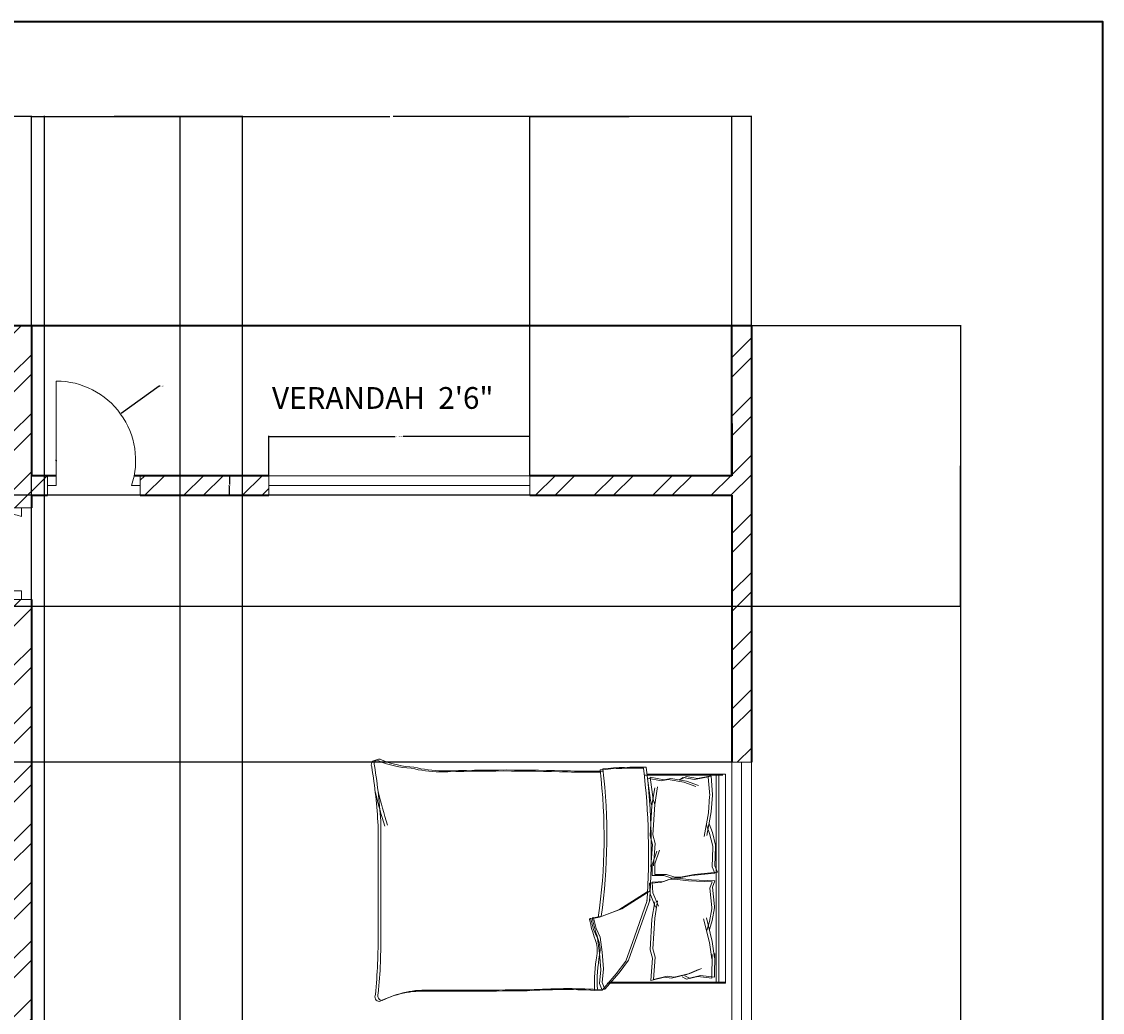
# Model space of a CAD drawing. Units: inches. Extents: x 2008 to 2657, y 1077 to 2165.
# Tile 16 of 16: x 2409 to 2657, y 1937 to 2165. Entities that reach past the tile are written whole.
import ezdxf

# ---------------------------------------------------------------- set-up
doc = ezdxf.new("R2010")
doc.units = ezdxf.units.IN
for name, color, linetype, lineweight in [('A-ANNO-DIMS', 2, 'Continuous', 18), ('A-ANNO-TTLB', 7, 'Continuous', 35), ('A-AREA-IDEN', 4, 'Continuous', 18), ('A-DOOR', 11, 'Continuous', 18), ('A-FURN', 8, 'Continuous', 13), ('A-GLAZ', 191, 'Continuous', 18), ('A-WALL', 7, 'Continuous', 35)]:
    doc.layers.add(name, color=color, linetype=linetype, lineweight=lineweight)
doc.layers.add('A-WALL-PATT', color=30, linetype='Continuous', lineweight=13, true_color=0xf8991e)
doc.styles.get("Standard").update_dxf_attribs({"font": 'arial.ttf'})
doc.dimstyles.get("Standard").update_dxf_attribs({"dimtxt": 0.18, "dimasz": 0.18, "dimexe": 0.18, "dimexo": 0.0625, "dimgap": 0.09, "dimtad": 0, "dimtih": 1, "dimtoh": 1, "dimdec": 4, "dimzin": 0, "dimdsep": 46, "dimtxsty": 'Standard', "dimcen": 0.09, "dimadec": 0, "dimazin": 0, "dimtfac": 1, "dimtdec": 4, "dimtofl": 0, "dimtmove": 0, "dimatfit": 3, "dimfxl": 1, "dimtolj": 1, "dimtzin": 0, "dimarcsym": 0})

# ---------------------------------------------------------------- blocks, each defined once
blk = doc.blocks.new('BED-DOUBLE')
for p, q in [((27.75, 52.87), (24.5, 49.16)), ((27.75, 52.87), (24.5, 49.16)), ((28.39, 53.1), (25.14, 49.39)), ((28.39, 53.1), (25.14, 49.39)), ((29.49, 52.95), (27.75, 52.87, 3.87)), ((29.49, 52.95), (27.75, 52.87, 3.87)), ((28.37, 51.33), (27.75, 52.87)), ((28.37, 51.33), (27.75, 52.87)), ((30.13, 53.18), (28.39, 53.1, 3.87)), ((30.13, 53.18), (28.39, 53.1, 3.87)), ((29, 51.56), (28.39, 53.1)), ((29, 51.56), (28.39, 53.1)), ((0, 51.49), (0.64, 51.49)), ((0, 3.48), (0, 51.49)), ((0, 51.27), (26.61, 51.27)), ((0, 51.27), (26.61, 51.27)), ((0.64, 51.49), (27.25, 51.49)), ((0.64, 51.49), (27.25, 51.49)), ((1.53, 3.48), (1.53, 51.27)), ((1.53, 3.48), (1.53, 51.27)), ((2.17, 3.7), (2.17, 51.49)), ((2.17, 3.7), (2.17, 51.49)), ((2.56, 50.11), (2.46, 44.71)), ((2.56, 50.11), (2.46, 44.71)), ((2.56, 50.11), (5.77, 49.73)), ((2.56, 50.11), (5.77, 49.73)), ((3.2, 50.34), (3.1, 44.94)), ((3.2, 50.34), (3.1, 44.94)), ((3.2, 50.34), (6.41, 49.96)), ((3.2, 50.34), (6.41, 49.96)), ((5.77, 49.73), (8.34, 50.33)), ((5.77, 49.73), (8.34, 50.33)), ((6.41, 49.96), (8.98, 50.56)), ((6.41, 49.96), (8.98, 50.56)), ((11.83, 50.11), (8.26, 49.31)), ((11.83, 50.11), (8.26, 49.31)), ((8.34, 50.33), (9.38, 49.82)), ((8.34, 50.33), (9.38, 49.81)), ((12.47, 50.34), (8.9, 49.54)), ((12.47, 50.34), (8.9, 49.54)), ((8.98, 50.56), (10.02, 50.04)), ((8.98, 50.56), (10.02, 50.04)), ((13.43, 49.92), (11.83, 50.11)), ((13.43, 49.92), (11.83, 50.11)), ((14.07, 50.15), (12.47, 50.34)), ((14.07, 50.15), (12.47, 50.34)), ((16.57, 50.7), (13.43, 49.92)), ((16.57, 50.7), (13.43, 49.92)), ((17.21, 50.93), (14.07, 50.15)), ((17.21, 50.93), (14.07, 50.15)), ((16.17, 45.57), (16.57, 50.7)), ((16.17, 45.57), (16.57, 50.7)), ((16.81, 45.8), (17.21, 50.93)), ((16.81, 45.8), (17.21, 50.93)), ((28.06, 48.23), (28.37, 51.33)), ((28.06, 48.23), (28.37, 51.33)), ((28.7, 48.46), (29, 51.56)), ((28.7, 48.46), (29, 51.56)), ((8.26, 49.31), (5.58, 48.13)), ((8.26, 49.31), (5.58, 48.13)), ((8.9, 49.54), (6.22, 48.36)), ((8.9, 49.54), (6.22, 48.36)), ((24.5, 49.16), (22.33, 46.22)), ((24.5, 49.16), (22.33, 46.22)), ((25.14, 49.39), (22.97, 46.45)), ((25.14, 49.39), (22.97, 46.45)), ((28.37, 44.36), (28.06, 48.23)), ((28.37, 44.36), (28.06, 48.23)), ((29, 44.59), (28.7, 48.46)), ((29, 44.59), (28.7, 48.46)), ((2.46, 44.71), (2.54, 45.71)), ((2.46, 44.71), (2.54, 45.71)), ((2.54, 45.71), (3.07, 41.91)), ((2.54, 45.71), (3.07, 41.91)), ((3.1, 44.94), (3.18, 45.94)), ((3.1, 44.94), (3.18, 45.94)), ((3.18, 45.94), (3.71, 42.14)), ((3.18, 45.94), (3.71, 42.14)), ((16.73, 43.61), (16.17, 45.57)), ((16.73, 43.61), (16.17, 45.57)), ((17.37, 43.84), (16.81, 45.8)), ((17.37, 43.83), (16.81, 45.8)), ((22.33, 46.22), (20.32, 40.64)), ((22.33, 46.22), (20.32, 40.64)), ((22.97, 46.45), (20.96, 40.87)), ((22.97, 46.45), (20.96, 40.87)), ((16.3, 36.6), (16.73, 43.61)), ((16.3, 36.6), (16.73, 43.61)), ((16.93, 36.83), (17.37, 43.84)), ((16.93, 36.82), (17.37, 43.83)), ((28.83, 40.95), (28.37, 44.36)), ((28.83, 40.95), (28.37, 44.36)), ((29.47, 41.18), (29, 44.59)), ((29.47, 41.18), (29, 44.59)), ((3.07, 41.91), (4.42, 36.5)), ((3.07, 41.91), (4.42, 36.5)), ((3.71, 42.14), (5.06, 36.72)), ((3.71, 42.14), (5.06, 36.72)), ((20.32, 40.64), (17.38, 32.31)), ((20.32, 40.64), (17.38, 32.31)), ((20.96, 40.87), (18.02, 32.54)), ((20.96, 40.87), (18.02, 32.53)), ((29.76, 38.94), (28.83, 40.95)), ((29.76, 38.94), (28.83, 40.95)), ((30.4, 39.17), (29.47, 41.18)), ((30.4, 39.17), (29.47, 41.18)), ((79.88, 15.29), (79.88, 39.91)), ((79.88, 15.29), (79.88, 39.91)), ((3.67, 39.2), (3.08, 37.14)), ((3.67, 39.2), (3.08, 37.14)), ((3.72, 37.36), (3.18, 34.43)), ((3.72, 37.36), (3.18, 34.43)), ((4.31, 39.43), (3.72, 37.36)), ((4.31, 39.43), (3.72, 37.36)), ((30.38, 36.46), (29.76, 38.94)), ((30.38, 36.46), (29.76, 38.94)), ((31.02, 36.69), (30.4, 39.17)), ((31.02, 36.69), (30.4, 39.17)), ((79.25, 15.06), (79.25, 39.68)), ((79.25, 15.06), (79.25, 39.68)), ((3.08, 37.14), (2.54, 34.21)), ((3.08, 37.14), (2.54, 34.2)), ((15.63, 32.56), (16.3, 36.6)), ((15.63, 32.56), (16.3, 36.6)), ((16.27, 32.79), (16.93, 36.83)), ((16.27, 32.79), (16.93, 36.82)), ((23.88, 34.45), (28.37, 36.15)), ((23.88, 34.45), (28.37, 36.15)), ((24.52, 34.68), (29, 36.38)), ((24.52, 34.68), (29, 36.38)), ((28.37, 36.15), (30.38, 36.46)), ((28.37, 36.15), (30.38, 36.46)), ((29, 36.38), (31.02, 36.69)), ((29, 36.38), (31.02, 36.69)), ((2.54, 34.21), (2.56, 33.88)), ((2.54, 34.2), (2.56, 33.88)), ((2.56, 33.88), (2.98, 29.46)), ((2.56, 33.88), (2.98, 29.46)), ((3.18, 34.43), (3.2, 34.11)), ((3.18, 34.43), (3.2, 34.11)), ((3.2, 34.11), (3.62, 29.68)), ((3.2, 34.11), (3.62, 29.68)), ((16.74, 30.75), (15.45, 33.82)), ((16.74, 30.75), (15.45, 33.82)), ((17.38, 30.98), (16.09, 34.05)), ((17.38, 30.98), (16.09, 34.05)), ((17.38, 30.26), (23.88, 34.45)), ((17.38, 30.26), (23.88, 34.45)), ((18.02, 30.49), (24.52, 34.68)), ((18.02, 30.49), (24.52, 34.68)), ((16.89, 28.3), (16.74, 30.75)), ((16.89, 28.3), (16.74, 30.75)), ((17.53, 28.53), (17.38, 30.98)), ((17.53, 28.53), (17.38, 30.98)), ((2.98, 29.46), (2.49, 27.98)), ((2.98, 29.46), (2.49, 27.98)), ((2.49, 27.98), (7.87, 27.73)), ((2.49, 27.98), (7.87, 27.73)), ((3.62, 29.68), (3.13, 28.21)), ((3.62, 29.68), (3.13, 28.21)), ((3.13, 28.21), (8.51, 27.96)), ((3.13, 28.21), (8.51, 27.96)), ((7.86, 26.79), (11.04, 27.37)), ((7.86, 26.79), (11.04, 27.37)), ((7.87, 27.73), (11.08, 27.36)), ((7.87, 27.73), (11.08, 27.36)), ((8.51, 27.96), (11.72, 27.58)), ((8.51, 27.96), (11.72, 27.58)), ((11.04, 27.37), (12.34, 27.37)), ((11.04, 27.37), (12.34, 27.37)), ((11.08, 27.36), (12.38, 27.44)), ((11.08, 27.36), (12.38, 27.44)), ((11.72, 27.58), (13.02, 27.66)), ((11.72, 27.58), (13.02, 27.66)), ((12.34, 27.37), (14.22, 26.79)), ((12.34, 27.37), (14.22, 26.79)), ((12.38, 27.44), (14.22, 28.13)), ((12.38, 27.44), (14.22, 28.13)), ((13.02, 27.66), (14.86, 28.36)), ((13.02, 27.66), (14.86, 28.36)), ((14.22, 28.13), (16.89, 28.3)), ((14.22, 28.13), (16.89, 28.3)), ((14.86, 28.36), (17.53, 28.53)), ((14.86, 28.36), (17.53, 28.53)), ((1.87, 25.98), (7.22, 26.56)), ((1.87, 25.98), (7.22, 26.56)), ((2.45, 24.54), (1.87, 25.98)), ((2.45, 24.54), (1.87, 25.98)), ((2.51, 26.21), (7.86, 26.79)), ((2.51, 26.21), (7.86, 26.79)), ((3.09, 24.77), (2.51, 26.21)), ((3.09, 24.77), (2.51, 26.21)), ((7.22, 26.56), (10.4, 27.14)), ((7.22, 26.56), (10.4, 27.14)), ((10.4, 27.14), (11.7, 27.14)), ((10.4, 27.14), (11.7, 27.14)), ((11.7, 27.14), (13.58, 26.56)), ((11.7, 27.14), (13.58, 26.56)), ((13.58, 26.56), (16.26, 26.56)), ((13.58, 26.56), (16.26, 26.56)), ((14.22, 26.79), (16.9, 26.79)), ((14.22, 26.79), (16.9, 26.79)), ((16.26, 26.56), (16.26, 24.1)), ((16.26, 26.56), (16.26, 24.1)), ((16.9, 26.79), (16.9, 24.33)), ((16.9, 26.79), (16.9, 24.33)), ((2.3, 20.09), (2.45, 24.54)), ((2.3, 20.09), (2.45, 24.54)), ((2.94, 20.32), (3.09, 24.77)), ((2.94, 20.32), (3.09, 24.77)), ((16.26, 24.1), (15.17, 20.96)), ((16.26, 24.1), (15.17, 20.96)), ((16.9, 24.33), (15.81, 21.19)), ((16.9, 24.33), (15.81, 21.19)), ((16.17, 19.38), (16.57, 24.52)), ((16.17, 19.38), (16.57, 24.52)), ((16.81, 19.61), (17.21, 24.74)), ((16.81, 19.61), (17.21, 24.74)), ((2.3, 19.77), (2.3, 20.09)), ((2.3, 19.77), (2.3, 20.09)), ((2.94, 20), (2.94, 20.32)), ((2.94, 20), (2.94, 20.32)), ((3.67, 17.11), (2.94, 20)), ((3.67, 17.11), (2.94, 20)), ((3.03, 16.88), (2.3, 19.77)), ((3.03, 16.88), (2.3, 19.77)), ((3.32, 12.11), (4.33, 17.6)), ((3.32, 12.11), (4.33, 17.6)), ((3.96, 12.34), (4.97, 17.83)), ((3.96, 12.34), (4.97, 17.83)), ((16.73, 17.42), (16.17, 19.38)), ((16.73, 17.42), (16.17, 19.38)), ((16.3, 10.41), (16.73, 17.42)), ((16.3, 10.41), (16.73, 17.42)), ((17.37, 17.65), (16.81, 19.61)), ((17.37, 17.65), (16.81, 19.61)), ((16.93, 10.64), (17.37, 17.65)), ((16.93, 10.64), (17.37, 17.65)), ((3.75, 14.86), (3.03, 16.88)), ((3.75, 14.86), (3.03, 16.88)), ((4.39, 15.08), (3.67, 17.11)), ((4.39, 15.08), (3.67, 17.11)), ((3.03, 8.29), (3.32, 12.11)), ((3.03, 8.29), (3.32, 12.11)), ((3.67, 8.51), (3.96, 12.34)), ((3.67, 8.51), (3.96, 12.34)), ((15.63, 6.38), (16.3, 10.41)), ((15.63, 6.38), (16.3, 10.41)), ((16.27, 6.61), (16.93, 10.64)), ((16.27, 6.61), (16.93, 10.64)), ((16.3, 10.41), (16.62, 9.28)), ((16.3, 10.41), (16.62, 9.28)), ((16.93, 10.64), (17.26, 9.51)), ((16.93, 10.64), (17.26, 9.51)), ((3.01, 8.18), (3.03, 8.29)), ((3.01, 8.18), (3.03, 8.29)), ((3.34, 3.9), (3.01, 8.18)), ((3.34, 3.9), (3.01, 8.18)), ((3.65, 8.41), (3.67, 8.51)), ((3.65, 8.41), (3.67, 8.51)), ((3.98, 4.13), (3.65, 8.41)), ((3.98, 4.13), (3.65, 8.41)), ((16.62, 9.28), (17.34, 4.18)), ((16.62, 9.28), (17.34, 4.18)), ((17.26, 9.51), (17.98, 4.41)), ((17.26, 9.51), (17.98, 4.41)), ((8.96, 5.05), (6.21, 6.06)), ((8.96, 5.05), (6.21, 6.06)), ((9.59, 5.28), (6.85, 6.29)), ((9.59, 5.28), (6.85, 6.29)), ((12.57, 4.47), (8.96, 5.05)), ((12.57, 4.47), (8.96, 5.05)), ((13.21, 4.7), (9.59, 5.28)), ((13.21, 4.7), (9.59, 5.28)), ((14.8, 4.99), (13.21, 4.7)), ((14.8, 4.99), (13.21, 4.7)), ((17.98, 4.41), (14.8, 4.99)), ((17.98, 4.41), (14.8, 4.99)), ((18.11, 3.48), (0, 3.48)), ((18.11, 3.48), (0, 3.48)), ((18.75, 3.7), (0.64, 3.7)), ((18.75, 3.7), (0.64, 3.7)), ((3.32, 3.9), (6.5, 4.47)), ((3.32, 3.89), (6.5, 4.47)), ((3.96, 4.12), (7.14, 4.7)), ((3.96, 4.12), (7.14, 4.7)), ((6.5, 4.47), (9.1, 4.04)), ((6.5, 4.47), (9.1, 4.04)), ((7.14, 4.7), (9.74, 4.27)), ((7.14, 4.7), (9.74, 4.27)), ((9.1, 4.04), (10.11, 4.62)), ((9.1, 4.04), (10.11, 4.62)), ((9.74, 4.27), (10.75, 4.85)), ((9.74, 4.27), (10.75, 4.85)), ((14.16, 4.76), (12.57, 4.47)), ((14.16, 4.76), (12.57, 4.47)), ((17.34, 4.18), (14.16, 4.76)), ((17.34, 4.18), (14.16, 4.76))]:
    blk.add_line(p, q)
for centre, radius, start, end in [((68.67, 76.16), 23.07, 267.4714, 296.4681), ((68.67, 76.16), 23.07, 267.4714, 296.4681), ((69.31, 76.39), 23.07, 267.4714, 296.4681), ((69.31, 76.39), 23.07, 267.4714, 296.4681), ((78.87, 54.41), 1.1, 332.6588, 86.02), ((78.87, 54.41), 1.1, 332.6588, 86.02), ((79.51, 54.64), 1.1, 332.6588, 86.02), ((79.51, 54.64), 1.1, 332.6588, 86.02), ((-6.66, 51.33), 36.18, 349.8763, 2.5657), ((-6.66, 51.33), 36.18, 349.8763, 2.5657), ((36.32, 182.27), 129.5, 266.9791, 273.8365), ((36.32, 182.27), 129.5, 266.9791, 273.8365), ((-6.02, 51.56), 36.18, 349.8763, 2.5657), ((-6.02, 51.56), 36.18, 349.8763, 2.5657), ((36.95, 182.49), 129.5, 266.9791, 273.8365), ((36.95, 182.49), 129.5, 266.9791, 273.8365), ((67.82, -4508.74), 4561.86, 90.00217, 90.28689), ((67.82, -4508.74), 4561.86, 90.00217, 90.28689), ((68.46, -4508.51), 4561.86, 90.00217, 90.28689), ((68.46, -4508.51), 4561.86, 90.00217, 90.28689), ((212.28, 41.15), 133.04, 174.4998, 180.6351), ((212.28, 41.15), 133.04, 174.4998, 180.6351), ((212.92, 41.38), 133.04, 174.4998, 180.6351), ((212.92, 41.38), 133.04, 174.4998, 180.6351), ((35.07, 43.74), 6.22, 168.6608, 203.7384), ((35.07, 43.74), 6.22, 168.6608, 203.7384), ((35.71, 43.97), 6.22, 168.6608, 203.7384), ((35.71, 43.97), 6.22, 168.6608, 203.7384), ((1.48, 31.15), 29.65, 10.6617, 19.8806), ((1.48, 31.15), 29.65, 10.6617, 19.8806), ((2.12, 31.38), 29.65, 10.6617, 19.8806), ((2.12, 31.38), 29.65, 10.6617, 19.8806), ((156.32, 17.76), 129.02, 171.7845, 186.9006), ((156.32, 17.76), 129.02, 171.7845, 186.9006), ((156.96, 17.98), 129.02, 171.7845, 186.9006), ((156.96, 17.98), 129.02, 171.7845, 186.9006), ((30.44, 36.64), 0.185, 250.2464, 1.1377), ((30.44, 36.64), 0.185, 250.2464, 1.1377), ((31.08, 36.87), 0.185, 250.2464, 1.1377), ((31.08, 36.86), 0.185, 250.2464, 1.1377), ((182.05, 21.36), 164.97, 176.0865, 186.7821), ((182.05, 21.36), 164.97, 176.0865, 186.7821), ((182.69, 21.59), 164.97, 176.0865, 186.7821), ((182.69, 21.59), 164.97, 176.0865, 186.7821), ((-23.71, -17.22), 106.46, 13.3832, 17.7053), ((-23.71, -17.22), 106.46, 13.3832, 17.7053), ((-23.07, -16.99), 106.46, 13.3832, 17.7053), ((-23.07, -16.99), 106.46, 13.3832, 17.7053), ((200.84, 21.43), 121.76, 182.9958, 189.4091), ((200.84, 21.43), 121.76, 182.9958, 189.4091), ((201.48, 21.66), 121.76, 182.9958, 189.4091), ((201.48, 21.66), 121.76, 182.9958, 189.4091), ((31.17, -167.31), 170.11, 88.4762, 91.0082), ((31.17, -167.31), 170.11, 88.4762, 91.0082), ((31.81, -167.08), 170.11, 88.4762, 91.0082), ((31.81, -167.08), 170.11, 88.4762, 91.0082), ((50.61, 484.82), 482.31, 268.2277, 271.7185), ((50.61, 484.82), 482.31, 268.2277, 271.7185), ((51.25, 485.05), 482.31, 268.2277, 271.7185), ((51.25, 485.05), 482.31, 268.2277, 271.7185), ((64.52, -26.9), 29.63, 76.0648, 88.9113), ((64.52, -26.9), 29.63, 76.0648, 88.9113), ((65.15, -26.67), 29.63, 76.0648, 88.9113), ((65.15, -26.67), 29.63, 76.0648, 88.9113), ((20.1, 85.16), 83.31, 268.7218, 275.604), ((20.1, 85.16), 83.31, 268.7218, 275.604), ((20.74, 85.39), 83.31, 268.7218, 275.604), ((20.74, 85.39), 83.31, 268.7218, 275.604), ((70.28, -21.66), 23.56, 67.9751, 86.652), ((70.28, -21.66), 23.56, 67.9751, 86.652), ((70.92, -21.43), 23.56, 67.9751, 86.652), ((70.92, -21.43), 23.56, 67.9751, 86.652), ((79.72, 1.09), 1.09, 236.1736, 23.4781), ((79.72, 1.09), 1.09, 236.1736, 23.4781), ((80.36, 1.32), 1.09, 236.1736, 23.4781), ((80.36, 1.32), 1.09, 236.1736, 23.4781)]:
    blk.add_arc(centre, radius, start, end)
blk = doc.blocks.new('WIN-60IN-B')
for p, q in [((0, 4.5), (0, 0)), ((0, 4.5), (60, 4.5)), ((60, 2.25), (60, 4.5)), ((60, 4.5), (60, 0)), ((0, 0), (0, 2.25)), ((0, 2.25), (60, 2.25)), ((60, 0), (0, 0))]:
    blk.add_line(p, q)
blk = doc.blocks.new('*D19')
at = {"layer": 'A-ANNO-DIMS', "color": 0, "lineweight": -2, "transparency": 16777216}
for p, q in [((2465.81, 2060.24), (2465.81, 2069.35)), ((2465.99, 2069.17), (2494.88, 2069.17)), ((2525.63, 2069.17), (2496.74, 2069.17)), ((2525.81, 2060.24), (2525.81, 2069.35))]:
    blk.add_line(p, q, dxfattribs=at)
at = {"layer": 'A-ANNO-DIMS', "color": 0, "transparency": 16777216}
for points in [[(2465.99, 2069.2), (2465.99, 2069.14), (2465.81, 2069.17)], [(2525.63, 2069.2), (2525.63, 2069.14), (2525.81, 2069.17)]]:
    blk.add_solid(points, dxfattribs=at)
at = {"layer": 'Defpoints', "color": 0, "transparency": 16777216}
for p in [(2465.81, 2069.17), (2465.81, 2060.17), (2525.81, 2060.17)]:
    blk.add_point(p, dxfattribs=at)
at = {"layer": 'A-ANNO-DIMS', "color": 0, "transparency": 16777216, "insert": (2495.81, 2069.17), "char_height": 0.18, "attachment_point": 5}
blk.add_mtext('\\A1;WIN B 60 TYP.', dxfattribs=at)
blk = doc.blocks.new('*D20')
at = {"layer": 'A-ANNO-DIMS', "color": 0, "lineweight": -2, "transparency": 16777216}
for p, q in [((2465.75, 2060.17), (2456.63, 2060.17)), ((2456.81, 2059.99), (2456.81, 2058.11)), ((2456.81, 2055.85), (2456.81, 2057.74)), ((2465.75, 2055.67), (2456.63, 2055.67))]:
    blk.add_line(p, q, dxfattribs=at)
at = {"layer": 'A-ANNO-DIMS', "color": 0, "transparency": 16777216}
for points in [[(2456.78, 2059.99), (2456.84, 2059.99), (2456.81, 2060.17)], [(2456.78, 2055.85), (2456.84, 2055.85), (2456.81, 2055.67)]]:
    blk.add_solid(points, dxfattribs=at)
at = {"layer": 'Defpoints', "color": 0, "transparency": 16777216}
for p in [(2465.81, 2060.17), (2456.81, 2055.67), (2465.81, 2055.67)]:
    blk.add_point(p, dxfattribs=at)
at = {"layer": 'A-ANNO-DIMS', "color": 0, "transparency": 16777216, "insert": (2456.81, 2057.92), "char_height": 0.18, "attachment_point": 5}
blk.add_mtext('\\A1;5 TYP.', dxfattribs=at)
blk = doc.blocks.new('*D32')
at = {"layer": 'A-ANNO-DIMS', "color": 0, "lineweight": -2, "transparency": 16777216}
for p, q in [((2576.82, 2094.67), (2624.99, 2094.67)), ((2624.81, 2094.49), (2624.81, 1641.86)), ((2624.81, 1188.85), (2624.81, 1641.49)), ((2576.82, 1188.67), (2624.99, 1188.67))]:
    blk.add_line(p, q, dxfattribs=at)
at = {"layer": 'A-ANNO-DIMS', "color": 0, "transparency": 16777216}
for points in [[(2624.78, 2094.49), (2624.84, 2094.49), (2624.81, 2094.67)], [(2624.78, 1188.85), (2624.84, 1188.85), (2624.81, 1188.67)]]:
    blk.add_solid(points, dxfattribs=at)
at = {"layer": 'Defpoints', "color": 0, "transparency": 16777216}
for p in [(2576.76, 2094.67), (2624.81, 2094.67), (2576.76, 1188.67)]:
    blk.add_point(p, dxfattribs=at)
at = {"layer": 'A-ANNO-DIMS', "color": 0, "transparency": 16777216, "insert": (2624.81, 1641.67), "char_height": 0.18, "attachment_point": 5}
blk.add_mtext('\\A1;906', dxfattribs=at)
blk = doc.blocks.new('*D36')
at = {"layer": 'A-ANNO-DIMS', "color": 0, "lineweight": -2, "transparency": 16777216}
for p, q in [((2318.26, 2094.74), (2318.26, 2142.9)), ((2318.44, 2142.72), (2364.54, 2142.72)), ((2411.08, 2142.72), (2364.98, 2142.72)), ((2411.26, 2094.74), (2411.26, 2142.9))]:
    blk.add_line(p, q, dxfattribs=at)
at = {"layer": 'A-ANNO-DIMS', "color": 0, "transparency": 16777216}
for points in [[(2318.44, 2142.75), (2318.44, 2142.69), (2318.26, 2142.72)], [(2411.08, 2142.75), (2411.08, 2142.69), (2411.26, 2142.72)]]:
    blk.add_solid(points, dxfattribs=at)
at = {"layer": 'Defpoints', "color": 0, "transparency": 16777216}
for p in [(2411.26, 2142.72), (2318.26, 2094.67), (2411.26, 2094.67)]:
    blk.add_point(p, dxfattribs=at)
at = {"layer": 'A-ANNO-DIMS', "color": 0, "transparency": 16777216, "insert": (2364.76, 2142.72), "char_height": 0.18, "attachment_point": 5}
blk.add_mtext('\\A1;93', dxfattribs=at)
blk = doc.blocks.new('*D37')
at = {"layer": 'A-ANNO-DIMS', "color": 0, "lineweight": -2, "transparency": 16777216}
for p, q in [((2411.26, 2094.74), (2411.26, 2142.9)), ((2411.44, 2142.72), (2493.63, 2142.72)), ((2576.58, 2142.72), (2494.4, 2142.72)), ((2576.76, 2094.74), (2576.76, 2142.9))]:
    blk.add_line(p, q, dxfattribs=at)
at = {"layer": 'A-ANNO-DIMS', "color": 0, "transparency": 16777216}
for points in [[(2411.44, 2142.75), (2411.44, 2142.69), (2411.26, 2142.72)], [(2576.58, 2142.75), (2576.58, 2142.69), (2576.76, 2142.72)]]:
    blk.add_solid(points, dxfattribs=at)
at = {"layer": 'Defpoints', "color": 0, "transparency": 16777216}
for p in [(2576.76, 2142.72), (2411.26, 2094.67), (2576.76, 2094.67)]:
    blk.add_point(p, dxfattribs=at)
at = {"layer": 'A-ANNO-DIMS', "color": 0, "transparency": 16777216, "insert": (2494.01, 2142.72), "char_height": 0.18, "attachment_point": 5}
blk.add_mtext('\\A1;165.5', dxfattribs=at)
blk = doc.blocks.new('*D49')
at = {"layer": 'A-ANNO-DIMS', "color": 0, "lineweight": -2, "transparency": 16777216}
for p, q in [((2250.82, 2094.67), (2624.99, 2094.67)), ((2624.81, 2094.49), (2624.81, 2062.61)), ((2624.81, 2030.35), (2624.81, 2062.24)), ((2250.82, 2030.17), (2624.99, 2030.17))]:
    blk.add_line(p, q, dxfattribs=at)
at = {"layer": 'A-ANNO-DIMS', "color": 0, "transparency": 16777216}
for points in [[(2624.78, 2094.49), (2624.84, 2094.49), (2624.81, 2094.67)], [(2624.78, 2030.35), (2624.84, 2030.35), (2624.81, 2030.17)]]:
    blk.add_solid(points, dxfattribs=at)
at = {"layer": 'Defpoints', "color": 0, "transparency": 16777216}
for p in [(2250.76, 2094.67), (2624.81, 2094.67), (2250.76, 2030.17)]:
    blk.add_point(p, dxfattribs=at)
at = {"layer": 'A-ANNO-DIMS', "color": 0, "transparency": 16777216, "insert": (2624.81, 2062.42), "char_height": 0.18, "attachment_point": 5}
blk.add_mtext('\\A1;64.5', dxfattribs=at)
blk = doc.blocks.new('*D56')
at = {"layer": 'A-ANNO-DIMS', "color": 0, "lineweight": -2, "transparency": 16777216}
for p, q in [((2411.26, 1842.83), (2411.26, 2142.9)), ((2411.44, 2142.72), (2435.18, 2142.72)), ((2459.58, 2142.72), (2435.84, 2142.72)), ((2459.76, 1830.56), (2459.76, 2142.9))]:
    blk.add_line(p, q, dxfattribs=at)
at = {"layer": 'A-ANNO-DIMS', "color": 0, "transparency": 16777216}
for points in [[(2411.44, 2142.75), (2411.44, 2142.69), (2411.26, 2142.72)], [(2459.58, 2142.75), (2459.58, 2142.69), (2459.76, 2142.72)]]:
    blk.add_solid(points, dxfattribs=at)
at = {"layer": 'Defpoints', "color": 0, "transparency": 16777216}
for p in [(2459.76, 2142.72), (2411.26, 1842.77), (2459.76, 1830.5)]:
    blk.add_point(p, dxfattribs=at)
at = {"layer": 'A-ANNO-DIMS', "color": 0, "transparency": 16777216, "insert": (2435.51, 2142.72), "char_height": 0.18, "attachment_point": 5}
blk.add_mtext('\\A1;48.5', dxfattribs=at)
blk = doc.blocks.new('*D57')
at = {"layer": 'A-ANNO-DIMS', "color": 0, "lineweight": -2, "transparency": 16777216}
for p, q in [((2414.28, 1754.24), (2414.28, 2142.9)), ((2414.46, 2142.72), (2429.47, 2142.72)), ((2445.27, 2142.72), (2430.26, 2142.72)), ((2445.45, 1751.99), (2445.45, 2142.9))]:
    blk.add_line(p, q, dxfattribs=at)
at = {"layer": 'A-ANNO-DIMS', "color": 0, "transparency": 16777216}
for points in [[(2414.46, 2142.75), (2414.46, 2142.69), (2414.28, 2142.72)], [(2445.27, 2142.75), (2445.27, 2142.69), (2445.45, 2142.72)]]:
    blk.add_solid(points, dxfattribs=at)
at = {"layer": 'Defpoints', "color": 0, "transparency": 16777216}
for p in [(2445.45, 2142.72), (2414.28, 1754.17), (2445.45, 1751.92)]:
    blk.add_point(p, dxfattribs=at)
at = {"layer": 'A-ANNO-DIMS', "color": 0, "transparency": 16777216, "insert": (2429.87, 2142.72), "char_height": 0.18, "attachment_point": 5}
blk.add_mtext('\\A1;31.17', dxfattribs=at)
blk = doc.blocks.new('*D60')
at = {"layer": 'A-ANNO-DIMS', "color": 0, "lineweight": -2, "transparency": 16777216}
for p, q in [((2525.81, 2060.24), (2525.81, 2142.9)), ((2525.99, 2142.72), (2548.64, 2142.72)), ((2572.08, 2142.72), (2549.43, 2142.72)), ((2572.26, 2060.24), (2572.26, 2142.9))]:
    blk.add_line(p, q, dxfattribs=at)
at = {"layer": 'A-ANNO-DIMS', "color": 0, "transparency": 16777216}
for points in [[(2525.99, 2142.75), (2525.99, 2142.69), (2525.81, 2142.72)], [(2572.08, 2142.75), (2572.08, 2142.69), (2572.26, 2142.72)]]:
    blk.add_solid(points, dxfattribs=at)
at = {"layer": 'Defpoints', "color": 0, "transparency": 16777216}
for p in [(2572.26, 2142.72), (2525.81, 2060.17), (2572.26, 2060.17)]:
    blk.add_point(p, dxfattribs=at)
at = {"layer": 'A-ANNO-DIMS', "color": 0, "transparency": 16777216, "insert": (2549.04, 2142.72), "char_height": 0.18, "attachment_point": 5}
blk.add_mtext('\\A1;46.45', dxfattribs=at)
blk = doc.blocks.new('*D66')
at = {"layer": 'A-ANNO-DIMS', "color": 0, "lineweight": -2, "transparency": 16777216}
for p, q in [((2572.2, 2055.67), (2028.03, 2055.67)), ((2028.21, 2055.49), (2028.21, 2025.16)), ((2028.21, 1994.47), (2028.21, 2024.8)), ((2572.2, 1994.29), (2028.03, 1994.29))]:
    blk.add_line(p, q, dxfattribs=at)
at = {"layer": 'A-ANNO-DIMS', "color": 0, "transparency": 16777216}
for points in [[(2028.18, 2055.49), (2028.24, 2055.49), (2028.21, 2055.67)], [(2028.18, 1994.47), (2028.24, 1994.47), (2028.21, 1994.29)]]:
    blk.add_solid(points, dxfattribs=at)
at = {"layer": 'Defpoints', "color": 0, "transparency": 16777216}
for p in [(2572.26, 2055.67), (2028.21, 1994.29), (2572.26, 1994.29)]:
    blk.add_point(p, dxfattribs=at)
at = {"layer": 'A-ANNO-DIMS', "color": 0, "transparency": 16777216, "insert": (2028.21, 2024.98), "char_height": 0.18, "attachment_point": 5}
blk.add_mtext('\\A1;61.39', dxfattribs=at)
blk = doc.blocks.new('*D84')
at = {"layer": 'A-ANNO-DIMS', "color": 0, "lineweight": -2, "transparency": 16777216}
for p, q in [((2440.65, 2080.74), (2431.93, 2074.46)), ((2440.83, 2080.74), (2440.65, 2080.74)), ((2416.9, 2063.7), (2417.08, 2063.7)), ((2416.99, 2063.61), (2416.99, 2063.79))]:
    blk.add_line(p, q, dxfattribs=at)
at = {"layer": 'A-ANNO-DIMS', "color": 0, "transparency": 16777216}
blk.add_solid([(2431.91, 2074.48), (2431.94, 2074.43), (2431.78, 2074.35)], dxfattribs=at)
at = {"layer": 'Defpoints', "color": 0, "transparency": 16777216}
for p in [(2431.78, 2074.35), (2416.99, 2063.7)]:
    blk.add_point(p, dxfattribs=at)
at = {"layer": 'A-ANNO-DIMS', "color": 0, "transparency": 16777216, "insert": (2441.31, 2080.74), "char_height": 0.18, "attachment_point": 5}
blk.add_mtext('\\A1;R18.23', dxfattribs=at)

msp = doc.modelspace()

# ---------------------------------------------------------------- hatches: boundary and pattern name
at = {"layer": 'A-WALL-PATT'}
h = msp.add_hatch(dxfattribs=at)
h.set_pattern_fill('ANSI32', color=256)
h.paths.add_polyline_path([(2109.2619, 2094.6743), (2104.7619, 2094.6743), (2104.7619, 2072.1743), (2104.7619, 2021.6151), (2109.2619, 2021.6151), (2109.2619, 2055.6743), (2126.1387, 2055.6743), (2126.1387, 2057.9243), (2126.1387, 2060.1743), (2109.2619, 2060.1743)])
h.paths.add_polyline_path([(2223.2494, 2057.9243), (2223.2494, 2060.1743), (2186.1387, 2060.1743), (2186.1387, 2055.6743), (2223.2494, 2055.6743)])
h.paths.add_polyline_path([(2250.7619, 2072.1743), (2250.7619, 2090.1743), (2250.7619, 2094.6743), (2246.2619, 2094.6743), (2246.2619, 2060.1743), (2242.7242, 2060.1743), (2242.7242, 2055.6743), (2246.2619, 2055.6743), (2246.2619, 1899.6743), (2242.7458, 1899.6743), (2242.7458, 1897.4243), (2242.7458, 1895.1743), (2246.2619, 1895.1743), (2246.2619, 1878.8745), (2248.5119, 1878.8745), (2250.7619, 1878.8745), (2250.7619, 1991.1743), (2250.7619, 2025.6743), (2257.6798, 2025.6743), (2257.6798, 2027.9243), (2257.6798, 2030.1743), (2250.7619, 2030.1743)])
h.paths.add_polyline_path([(2411.2619, 2031.6743), (2409.0119, 2031.6743), (2406.7619, 2031.6743), (2406.7619, 2030.1743), (2322.7619, 2030.1743), (2322.7619, 2053.3443), (2318.2619, 2053.3443), (2318.2619, 2030.1743), (2305.6798, 2030.1743), (2305.6798, 2025.6743), (2318.2619, 2025.6743), (2322.7619, 2025.6743), (2406.7619, 2025.6743), (2406.7619, 1995.6743), (2406.7619, 1847.2677), (2250.7619, 1847.2677), (2250.7619, 1850.9902), (2248.5119, 1850.9902), (2246.2619, 1850.9902), (2246.2619, 1847.1743), (2246.2619, 1842.7677), (2303.0015, 1842.7677), (2303.0015, 1667.2413), (2298.4208, 1667.2413), (2298.4208, 1662.7413), (2303.0015, 1662.7413), (2303.0015, 1649.8758), (2307.5015, 1649.8758), (2307.5015, 1842.7677), (2406.7619, 1842.7677), (2411.2619, 1842.7677), (2411.2619, 1878.6743), (2415.8196, 1878.6743), (2415.8196, 1880.9243), (2415.8196, 1883.1743), (2411.2619, 1883.1743)])
h.paths.add_polyline_path([(2411.2619, 2094.6743), (2406.7619, 2094.6743), (2318.2619, 2094.6743), (2318.2619, 2077.3443), (2322.7619, 2077.3443), (2322.7619, 2090.1743), (2406.7619, 2090.1743), (2406.7619, 2072.1743), (2406.7619, 2067.6743), (2406.7619, 2052.7524), (2411.2619, 2052.7524), (2411.2619, 2055.6743), (2414.9888, 2055.6743), (2414.9888, 2057.9243), (2414.9888, 2060.1743), (2411.2619, 2060.1743), (2411.2619, 2072.1743)])
h.paths.add_polyline_path([(2576.7619, 2072.1743), (2576.7619, 2094.6743), (2572.2619, 2094.6743), (2572.2619, 2060.1743), (2525.8113, 2060.1743), (2525.8113, 2055.6743), (2572.2619, 2055.6743), (2572.2619, 1994.289), (2576.7619, 1994.289)])
h.paths.add_polyline_path([(2465.8113, 2060.1743), (2436.2802, 2060.1743), (2436.2802, 2055.6743), (2465.8113, 2055.6743), (2465.8113, 2057.9243)])
h.paths.add_polyline_path([(2576.7619, 1934.289), (2574.5119, 1934.289), (2572.2619, 1934.289), (2572.2619, 1883.1743), (2447.7027, 1883.1743), (2447.7027, 1878.6743), (2459.7619, 1878.6743), (2459.7619, 1830.4982), (2464.2619, 1830.4982), (2464.2619, 1878.6743), (2572.2619, 1878.6743), (2572.2619, 1868.4883), (2576.7619, 1868.4883)])
h.paths.add_polyline_path([(2576.7619, 1832.4883), (2572.2619, 1832.4883), (2572.2619, 1806.6743), (2464.2619, 1806.6743), (2464.2619, 1809.6629), (2459.7619, 1809.6629), (2459.7619, 1802.1743), (2483.7619, 1802.1743), (2483.7619, 1778.1743), (2488.2619, 1778.1743), (2488.2619, 1802.1743), (2572.2619, 1802.1743), (2572.2619, 1793.6101), (2576.7619, 1793.6101)])
h.paths.add_polyline_path([(2576.7619, 1769.6101), (2572.2619, 1769.6101), (2572.2619, 1754.1743), (2488.2619, 1754.1743), (2488.2619, 1757.2675), (2486.0119, 1757.2675), (2483.7619, 1757.2675), (2483.7619, 1754.1743), (2447.4528, 1754.1743), (2447.4528, 1749.6743), (2483.7619, 1749.6743), (2572.2619, 1749.6743), (2572.2619, 1715.1837), (2576.7619, 1715.1837)])
h.paths.add_polyline_path([(2576.7619, 1655.1837), (2572.2619, 1655.1837), (2572.2619, 1617.6743), (2411.2619, 1617.6743), (2411.2619, 1749.6743), (2414.2827, 1749.6743), (2414.2827, 1754.1743), (2406.7619, 1754.1743), (2406.7619, 1749.6743), (2406.7619, 1617.6743), (2307.5015, 1617.6743), (2307.5015, 1621.0007), (2305.2515, 1621.0007), (2303.0015, 1621.0007), (2303.0015, 1609.6944), (2307.5015, 1609.6944), (2307.5015, 1613.1743), (2406.7619, 1613.1743), (2406.7619, 1476.6743), (2415.532, 1476.6743), (2415.532, 1478.9243), (2415.532, 1481.1743), (2411.2619, 1481.1743), (2411.2619, 1613.1743), (2572.2619, 1613.1743), (2572.2619, 1584.6086), (2576.7619, 1584.6086)])
h.paths.add_polyline_path([(2576.7619, 1524.6086), (2572.2619, 1524.6086), (2572.2619, 1481.1743), (2483.7619, 1481.1743), (2447.5119, 1481.1743), (2447.5119, 1476.6743), (2483.7619, 1476.6743), (2483.7619, 1473.5051), (2488.2619, 1473.5051), (2488.2619, 1476.6743), (2572.2619, 1476.6743), (2572.2619, 1469.5488), (2576.7619, 1469.5488)])
h.paths.add_polyline_path([(2576.7619, 1445.5488), (2572.2619, 1445.5488), (2572.2619, 1428.6743), (2488.2619, 1428.6743), (2488.2619, 1455.6743), (2486.0119, 1455.6743), (2483.7619, 1455.6743), (2483.7619, 1428.6743), (2459.7619, 1428.6743), (2459.7619, 1422.1519), (2464.2619, 1422.1519), (2464.2619, 1424.1743), (2572.2619, 1424.1743), (2572.2619, 1407.5685), (2576.7619, 1407.5685)])
h.paths.add_polyline_path([(2576.7619, 1371.5685), (2572.2619, 1371.5685), (2572.2619, 1352.1743), (2464.2619, 1352.1743), (2464.2619, 1403.1384), (2462.0119, 1403.1384), (2459.7619, 1403.1384), (2459.7619, 1352.1743), (2446.3194, 1352.1743), (2446.3194, 1347.6743), (2572.2619, 1347.6743), (2572.2619, 1321.0291), (2576.7619, 1321.0291)])
h.paths.add_polyline_path([(2462.703, 1227.6743), (2436.0298, 1227.6743), (2436.0298, 1225.4243), (2436.0298, 1223.1743), (2462.703, 1223.1743), (2462.703, 1225.4243)])
h.paths.add_polyline_path([(2576.7619, 1261.0291), (2574.5119, 1261.0291), (2572.2619, 1261.0291), (2572.2619, 1227.6743), (2522.703, 1227.6743), (2522.703, 1223.1743), (2572.2619, 1223.1743), (2572.2619, 1188.6743), (2576.7619, 1188.6743), (2576.7619, 1193.1743), (2576.7619, 1223.1743)])
h.paths.add_polyline_path([(2414.2823, 1227.6743), (2411.2619, 1227.6743), (2411.2619, 1267.1779), (2409.0119, 1267.1779), (2406.7619, 1267.1779), (2406.7619, 1227.6743), (2322.7619, 1227.6743), (2322.7619, 1244.3623), (2318.2619, 1244.3623), (2318.2619, 1223.1743), (2406.7619, 1223.1743), (2406.7619, 1193.1743), (2406.7619, 1188.6743), (2411.2619, 1188.6743), (2411.2619, 1193.1743), (2411.2619, 1223.1743), (2414.2823, 1223.1743)])
h.paths.add_polyline_path([(2411.2619, 1347.6743), (2414.702, 1347.6743), (2414.702, 1349.9243), (2414.702, 1352.1743), (2411.2619, 1352.1743), (2411.2619, 1416.7413), (2307.5015, 1416.7413), (2307.5015, 1579.8489), (2305.2515, 1579.8489), (2303.0015, 1579.8489), (2303.0015, 1566.7413), (2299.2719, 1566.7413), (2299.2719, 1562.2413), (2303.0015, 1562.2413), (2303.0015, 1416.7413), (2246.2619, 1416.7413), (2246.2619, 1409.8616), (2250.7619, 1409.8616), (2250.7619, 1412.2413), (2406.7619, 1412.2413), (2406.7619, 1292.1743), (2304.9703, 1292.1743), (2304.9703, 1287.6743), (2318.2619, 1287.6743), (2318.2619, 1268.3623), (2322.7619, 1268.3623), (2322.7619, 1287.6743), (2406.7619, 1287.6743), (2406.7619, 1285.4748), (2411.2619, 1285.4748)])
h.paths.add_polyline_path([(2109.2619, 1262.7482), (2104.7619, 1262.7482), (2104.7619, 1223.1743), (2104.7619, 1193.1743), (2104.7619, 1188.6743), (2109.2619, 1188.6743), (2109.2619, 1223.1743), (2126.7928, 1223.1743), (2126.7928, 1225.4243), (2126.7928, 1227.6743), (2109.2619, 1227.6743)])
h.paths.add_polyline_path([(2222.3268, 1227.6743), (2186.7928, 1227.6743), (2186.7928, 1223.1743), (2222.3268, 1223.1743)])
h.paths.add_polyline_path([(2250.7619, 1287.6743), (2256.9703, 1287.6743), (2256.9703, 1289.9243), (2256.9703, 1292.1743), (2250.7619, 1292.1743), (2250.7619, 1382.2078), (2248.5119, 1382.2078), (2246.2619, 1382.2078), (2246.2619, 1347.6743), (2246.2619, 1227.6743), (2242.6068, 1227.6743), (2242.6068, 1223.1743), (2246.2619, 1223.1743), (2246.2619, 1188.6743), (2250.7619, 1188.6743), (2250.7619, 1193.1743), (2250.7619, 1227.6743)])
h.paths.add_polyline_path([(2133.2619, 1349.9243), (2133.2619, 1352.1743), (2109.2619, 1352.1743), (2109.2619, 1375.2826), (2104.7619, 1375.2826), (2104.7619, 1322.7482), (2109.2619, 1322.7482), (2109.2619, 1347.6743), (2133.2619, 1347.6743)])
h.paths.add_polyline_path([(2210.2105, 1352.1743), (2161.7619, 1352.1743), (2161.7619, 1412.2413), (2185.7619, 1412.2413), (2185.7619, 1420.1851), (2183.5119, 1420.1851), (2181.2619, 1420.1851), (2181.2619, 1416.7413), (2109.2619, 1416.7413), (2109.2619, 1452.4006), (2104.7619, 1452.4006), (2104.7619, 1399.2826), (2109.2619, 1399.2826), (2109.2619, 1412.2413), (2157.2619, 1412.2413), (2157.2619, 1352.1743), (2154.3383, 1352.1743), (2154.3383, 1347.6743), (2210.2105, 1347.6743)])
h.paths.add_polyline_path([(2185.7619, 1514.2413), (2161.7619, 1514.2413), (2161.7619, 1518.1307), (2159.5119, 1518.1307), (2157.2619, 1518.1307), (2157.2619, 1514.2413), (2109.2619, 1514.2413), (2109.2619, 1528.997), (2107.0119, 1528.997), (2104.7619, 1528.997), (2104.7619, 1488.4006), (2109.2619, 1488.4006), (2109.2619, 1509.7413), (2181.2619, 1509.7413), (2181.2619, 1441.2042), (2185.7619, 1441.2042)])
h.paths.add_polyline_path([(2270.4025, 1566.7413), (2109.2619, 1566.7413), (2080.7619, 1566.7413), (2080.7619, 1586.5643), (2076.2619, 1586.5643), (2076.2619, 1562.2413), (2080.7619, 1562.2413), (2104.7619, 1562.2413), (2104.7619, 1552.997), (2109.2619, 1552.997), (2109.2619, 1562.2413), (2157.2619, 1562.2413), (2157.2619, 1538.2413), (2161.7619, 1538.2413), (2161.7619, 1562.2413), (2205.2619, 1562.2413), (2270.4025, 1562.2413)])
h.paths.add_polyline_path([(2131.6813, 1897.4243), (2131.6813, 1899.6743), (2109.2619, 1899.6743), (2109.2619, 1961.6151), (2104.7619, 1961.6151), (2104.7619, 1886.8042), (2109.2619, 1886.8042), (2109.2619, 1895.1743), (2131.6813, 1895.1743)])
h.paths.add_polyline_path([(2185.7619, 1847.1743), (2161.7619, 1847.1743), (2161.7619, 1895.1743), (2185.7619, 1895.1743), (2211.543, 1895.1743), (2211.543, 1897.4243), (2211.543, 1899.6743), (2154.0916, 1899.6743), (2154.0916, 1897.4243), (2154.0916, 1895.1743), (2157.2619, 1895.1743), (2157.2619, 1847.1743), (2109.2619, 1847.1743), (2109.2619, 1862.8042), (2104.7619, 1862.8042), (2104.7619, 1821.243), (2109.2619, 1821.243), (2109.2619, 1842.6743), (2181.2619, 1842.6743), (2181.2619, 1840.6763), (2185.7619, 1840.6763)])
h.paths.add_polyline_path([(2109.2619, 1785.243), (2104.7619, 1785.243), (2104.7619, 1715.4691), (2109.2619, 1715.4691), (2109.2619, 1730.8423), (2157.2619, 1730.8423), (2157.2619, 1727.6404), (2161.7619, 1727.6404), (2161.7619, 1730.8423), (2185.7619, 1730.8423), (2185.7619, 1822.1438), (2183.5119, 1822.1438), (2181.2619, 1822.1438), (2181.2619, 1735.3423), (2109.2619, 1735.3423)])
h.paths.add_polyline_path([(2109.2619, 1691.4691), (2104.7619, 1691.4691), (2104.7619, 1667.2413), (2076.2619, 1667.2413), (2076.2619, 1646.5643), (2080.7619, 1646.5643), (2080.7619, 1662.7413), (2109.2619, 1662.7413), (2271.4941, 1662.7413), (2271.4941, 1664.9913), (2271.4941, 1667.2413), (2181.2619, 1667.2413), (2161.7619, 1667.2413), (2161.7619, 1708.3752), (2159.5119, 1708.3752), (2157.2619, 1708.3752), (2157.2619, 1667.2413), (2109.2619, 1667.2413)])
h.paths.add_polyline_path([(2233.1467, 1747.4973), (2270.0737, 1747.4973), (2270.0737, 1766.1547), (2233.1467, 1766.1547)], flags=9)

# ---------------------------------------------------------------- linework, layer by layer
at = {"layer": 'A-ANNO-TTLB'}
msp.add_lwpolyline([(2008.4537, 2164.5615), (2657.4477, 2164.5615), (2657.4477, 1076.8888), (2008.4537, 1076.8888)], close=True, dxfattribs=at)
at = {"layer": 'A-DOOR'}
for p, q in [((2416.9888, 2057.9243), (2416.9888, 2081.9243)), ((2414.9888, 2060.1743), (2414.9888, 2055.6743)), ((2436.2802, 2060.1743), (2436.2802, 2055.6743)), ((2414.9888, 2055.6743), (2414.9888, 2057.9243)), ((2414.9888, 2057.9243), (2416.9888, 2057.9243)), ((2436.2802, 2057.9243), (2434.2802, 2057.9243)), ((2436.2802, 2055.6743), (2436.2802, 2057.9243)), ((2406.7619, 2052.7524), (2411.2619, 2052.7524)), ((2411.2619, 2052.7524), (2409.0119, 2052.7524)), ((2409.0119, 2052.7524), (2409.0119, 2050.7524)), ((2409.0119, 2033.6743), (2385.0119, 2033.6743)), ((2409.0119, 2031.6743), (2409.0119, 2033.6743)), ((2406.7619, 2031.6743), (2411.2619, 2031.6743)), ((2411.2619, 2031.6743), (2409.0119, 2031.6743))]:
    msp.add_line(p, q, dxfattribs=at)
for centre, radius, start, end in [((2416.9888, 2063.6954), 18.2289, 341.543346, 90), ((2403.0881, 2033.6743), 18.0762, 70.87007, 180)]:
    msp.add_arc(centre, radius, start, end, dxfattribs=at)
at = {"layer": 'A-WALL'}
for p, q in [((2406.7619, 2094.6743), (2572.2619, 2094.6743)), ((2411.2619, 2094.6743), (2411.2619, 2072.1743)), ((2572.2619, 2060.1743), (2572.2619, 2094.6743)), ((2572.2619, 2094.6743), (2576.7619, 2094.6743)), ((2576.7619, 2094.6743), (2576.7619, 2072.1743)), ((2411.2619, 2072.1743), (2411.2619, 2060.1743)), ((2572.2619, 2072.1743), (2572.2619, 2060.1743)), ((2576.7619, 2072.1743), (2576.7619, 1994.289)), ((2416.9888, 2060.1743), (2411.2619, 2060.1743)), ((2465.8113, 2060.1743), (2434.8745, 2060.1743)), ((2572.2619, 2060.1743), (2525.8113, 2060.1743)), ((2411.2619, 2055.6743), (2414.9888, 2055.6743)), ((2411.2619, 2055.6743), (2411.2619, 2052.7524)), ((2436.2802, 2055.6743), (2465.8113, 2055.6743)), ((2525.8113, 2055.6743), (2572.2619, 2055.6743)), ((2572.2619, 2055.6743), (2572.2619, 1994.289)), ((2411.2619, 2031.6743), (2411.2619, 1883.1743))]:
    msp.add_line(p, q, dxfattribs=at)

# ---------------------------------------------------------------- block references
at = {"layer": 'A-FURN', "rotation": 180}
msp.add_blockref('BED-DOUBLE', (2570.8423, 1995.0213), dxfattribs=at)
at = {"layer": 'A-GLAZ'}
for p, rotation in [((2525.811, 2060.1747), 180), ((2572.2616, 1994.2888), 270.0000000000001)]:
    msp.add_blockref('WIN-60IN-B', p, dxfattribs=dict(at, rotation=rotation))

# ---------------------------------------------------------------- texts
at = {"layer": 'A-AREA-IDEN', "insert": (2466.567, 2080.5405), "char_height": 5, "attachment_point": 1}
msp.add_mtext_dynamic_manual_height_columns('VERANDAH  2\'6"', width=184.353075, gutter_width=12.5, heights=[0], dxfattribs=at)

# ---------------------------------------------------------------- dimensions: what is measured, and where the dimension line sits
at = {"layer": 'A-ANNO-DIMS'}
for base, p1, p2, override, picture, middle in [((2411.2619, 2142.7243), (2318.2619, 2094.6743), (2411.2619, 2094.6743), {"dimdec": 0, "dimlfac": 1, "dimrnd": 0, "dimzin": 0, "dimdsep": 46, "dimlunit": 2}, '*D36', (2364.7619, 2142.7243)), ((2576.7619, 2142.7243), (2411.2619, 2094.6743), (2576.7619, 2094.6743), {"dimdec": 1, "dimlfac": 1, "dimrnd": 0, "dimzin": 0, "dimdsep": 46, "dimlunit": 2}, '*D37', (2494.0119, 2142.7243)), ((2459.7619, 2142.7243), (2411.2619, 1842.7677), (2459.7619, 1830.4982), {"dimdec": 1, "dimlfac": 1, "dimrnd": 0, "dimzin": 0, "dimdsep": 46, "dimlunit": 2}, '*D56', (2435.5119, 2142.7243)), ((2445.4528, 2142.7243), (2414.2827, 1754.1743), (2445.4528, 1751.9243), {"dimdec": 2, "dimlfac": 1, "dimrnd": 0, "dimzin": 0, "dimdsep": 46, "dimlunit": 2}, '*D57', (2429.8677, 2142.7243)), ((2572.2619, 2142.7243), (2525.8113, 2060.1743), (2572.2619, 2060.1743), {"dimdec": 2, "dimlfac": 1, "dimrnd": 0, "dimzin": 0, "dimdsep": 46, "dimlunit": 2}, '*D60', (2549.0366, 2142.7243))]:
    dim = msp.add_linear_dim(base=base, p1=p1, p2=p2, dimstyle='Standard', override=override, dxfattribs=at)
    dim.commit()
    dim.dimension.update_dxf_attribs({"geometry": picture, "text_midpoint": middle})
for base, p1, p2, override, picture, middle in [((2624.8119, 2094.6743), (2250.7619, 2030.1743), (2250.7619, 2094.6743), {"dimdec": 1, "dimlfac": 1, "dimrnd": 0, "dimzin": 0, "dimdsep": 46, "dimlunit": 2}, '*D49', (2624.8119, 2062.4243)), ((2624.8119, 2094.6743), (2576.7619, 1188.6743), (2576.7619, 2094.6743), {"dimdec": 0, "dimlfac": 1, "dimrnd": 0, "dimzin": 0, "dimdsep": 46, "dimlunit": 2}, '*D32', (2624.8119, 1641.6743)), ((2028.2119, 1994.289), (2572.2619, 2055.6743), (2572.2619, 1994.289), {"dimdec": 2, "dimlfac": 1, "dimrnd": 0, "dimzin": 0, "dimdsep": 46, "dimlunit": 2}, '*D66', (2028.2119, 2024.9817))]:
    dim = msp.add_linear_dim(base=base, p1=p1, p2=p2, angle=90, dimstyle='Standard', override=override, dxfattribs=at)
    dim.commit()
    dim.dimension.update_dxf_attribs({"geometry": picture, "text_midpoint": middle})
dim = msp.add_radius_dim(center=(2416.9888, 2063.6954), mpoint=(2431.7791, 2074.3511), dimstyle='Standard', override={"dimdec": 2, "dimlfac": 1, "dimrnd": 0, "dimzin": 0, "dimdsep": 46, "dimlunit": 2}, dxfattribs=at)
dim.commit()
dim.dimension.update_dxf_attribs({"geometry": '*D84', "text_midpoint": (2441.3131, 2080.7445), "dimtype": 164})
for base, p1, p2, angle, text, picture, middle in [((2465.8113, 2069.1743), (2525.8113, 2060.1743), (2465.8113, 2060.1743), 180, 'WIN B <> TYP.', '*D19', (2495.8113, 2069.1743)), ((2456.8113061011, 2055.6743446228), (2465.8113061011, 2060.1743446228), (2465.8113061011, 2055.6743446228), 270, '<> TYP.', '*D20', (2456.8113061011, 2057.9243446228))]:
    dim = msp.add_linear_dim(base=base, p1=p1, p2=p2, angle=angle, text=text, dimstyle='Standard', override={"dimdec": 0, "dimlfac": 1, "dimrnd": 0, "dimzin": 0, "dimdsep": 46, "dimlunit": 2}, dxfattribs=at)
    dim.commit()
    dim.dimension.update_dxf_attribs({"geometry": picture, "text_midpoint": middle})

doc.saveas('drawing.dxf')
